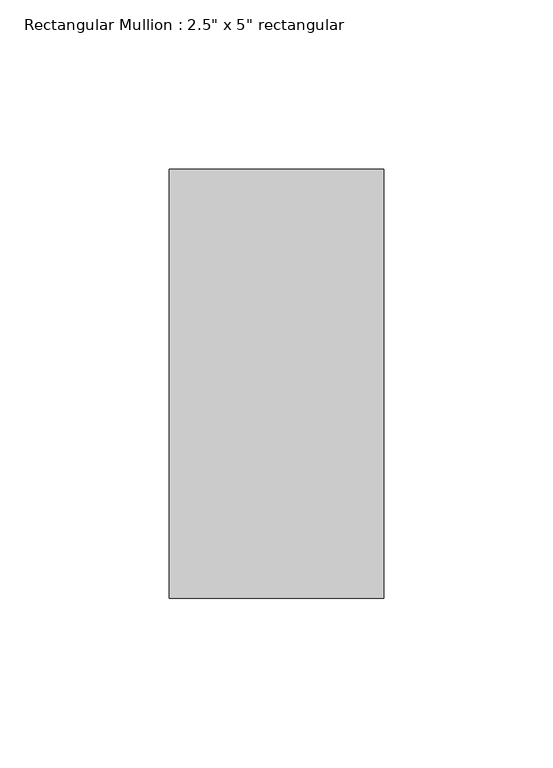
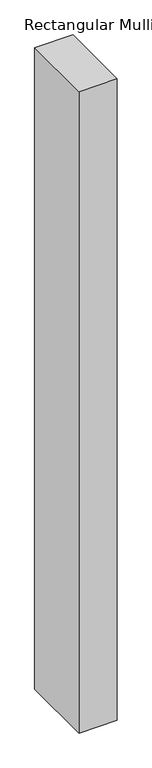
"""IFC4 building model written with IfcOpenShell, lengths in millimetres: member geometry."""

from ifc_helpers import new_model, si_unit, frame, origin, place, context, project, spatial, polyline, outline, extrude, source, transform, mapped, element, save


def member_e6b9f524(model_context):
    return source(origin(), model_context, "Body", "SweptSolid", [
        extrude(outline(polyline([(0.0, 63.5), (0.0, -63.5), (-63.5, -63.5), (-63.5, 63.5), (0.0, 63.5)])), frame((0.0, 0.0, -1123.95), z_axis=(0.0, 0.0, 1.0), x_axis=(1.0, 0.0, 0.0)), (0.0, 0.0, 1.0), 1123.95),
    ])


if __name__ == "__main__":
    model = new_model("IFC4")
    model_context = context("Model", 3, world=origin())
    ifc_project = project(units=[si_unit("LENGTHUNIT", "METRE", prefix="MILLI")], contexts=[model_context])
    site = spatial("IfcSite", under=ifc_project)
    building = spatial("IfcBuilding", under=site)
    placement = place(None, origin())
    member_shape = member_e6b9f524(model_context)
    element("IfcMember", 1, ObjectType="Rectangular Mullion : 2.5\" x 5\" rectangular", at=placement, inside=building, context=model_context, shape_type="MappedRepresentation", body=[
        mapped(member_shape, transform((0.0, 0.0, 0.0), x_axis=(1.0, 0.0, 0.0), y_axis=(0.0, 1.0, 0.0), z_axis=(0.0, 0.0, 1.0))),
    ])
    save(model, "model.ifc")

# Revit data of these elements
# Type "Rectangular Mullion : 2.5\" x 5\" rectangular"
#   built-in parameter 1007304 = 0.416667 (stored number, unit not read)
#   built-in parameter 1007301 = 0.104167 (stored number, unit not read)
#   built-in parameter 1007300 = 0.104167 (stored number, unit not read)
# Element 1 (IfcMember, "Rectangular Mullion : 2.5\" x 5\" rectangular")
#   Materials on its faces: "Aluminum"
# Materials
#   "Aluminum": class "Metal", colour RGB 247 247 247, transparency 0, Description = "Aluminum 6061", Cost = 0
